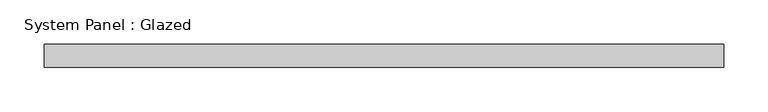
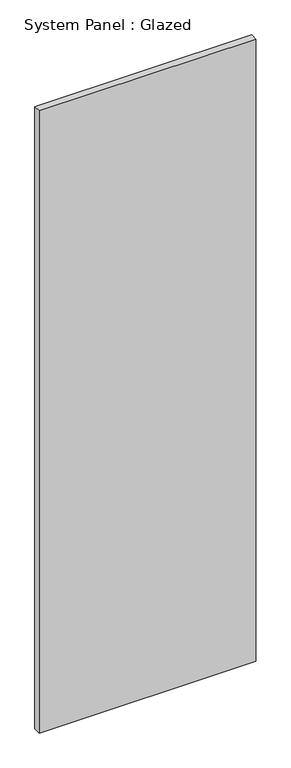
"""IFC4 building model written with IfcOpenShell, lengths in millimetres: plate geometry, System Panel : Glazed."""

from ifc_helpers import new_model, si_unit, origin, origin_with_axes, place, context, project, spatial, polyline, outline, extrude, source, transform, mapped, element, save


def system_panel_glazed_973f3ce5(model_context):
    return source(origin(), model_context, "Body", "SweptSolid", [
        extrude(outline(polyline([(382.0583333, 19.05), (-382.0583333, 19.05), (-382.0583333, 44.45), (382.0583333, 44.45), (382.0583333, 19.05)])), origin_with_axes(), (0.0, 0.0, 1.0), 2317.75),
    ])


if __name__ == "__main__":
    model = new_model("IFC4")
    model_context = context("Model", 3, world=origin())
    ifc_project = project(units=[si_unit("LENGTHUNIT", "METRE", prefix="MILLI")], contexts=[model_context])
    site = spatial("IfcSite", under=ifc_project)
    building = spatial("IfcBuilding", under=site)
    placement = place(None, origin())
    system_panel_glazed_shape = system_panel_glazed_973f3ce5(model_context)
    element("IfcPlate", 1, ObjectType="System Panel : Glazed", at=placement, inside=building, context=model_context, shape_type="MappedRepresentation", body=[
        mapped(system_panel_glazed_shape, transform((0.0, 0.0, 0.0), x_axis=(1.0, 0.0, 0.0), y_axis=(0.0, 1.0, 0.0), z_axis=(0.0, 0.0, 1.0))),
    ])
    save(model, "model.ifc")

# Revit data of these elements
# Type "System Panel : Glazed"
#   Construction Type Id = "GSP4R"
#   Analytic Construction = "1/8 in Pilkington single glazing"
#   Visual Light Transmittance = 0.9
#   Solar Heat Gain Coefficient = 0.86
#   Heat Transfer Coefficient (U) = 1.18115 BTU/(h·ft²·°F)
# Element 1 (IfcPlate, "System Panel : Glazed")
#   Materials on its faces: "Glass"
# Materials
#   "Glass": class "Glass", colour RGB 0 128 192, transparency 0.75, Description = "Soda Lime Glass", Cost = 0
